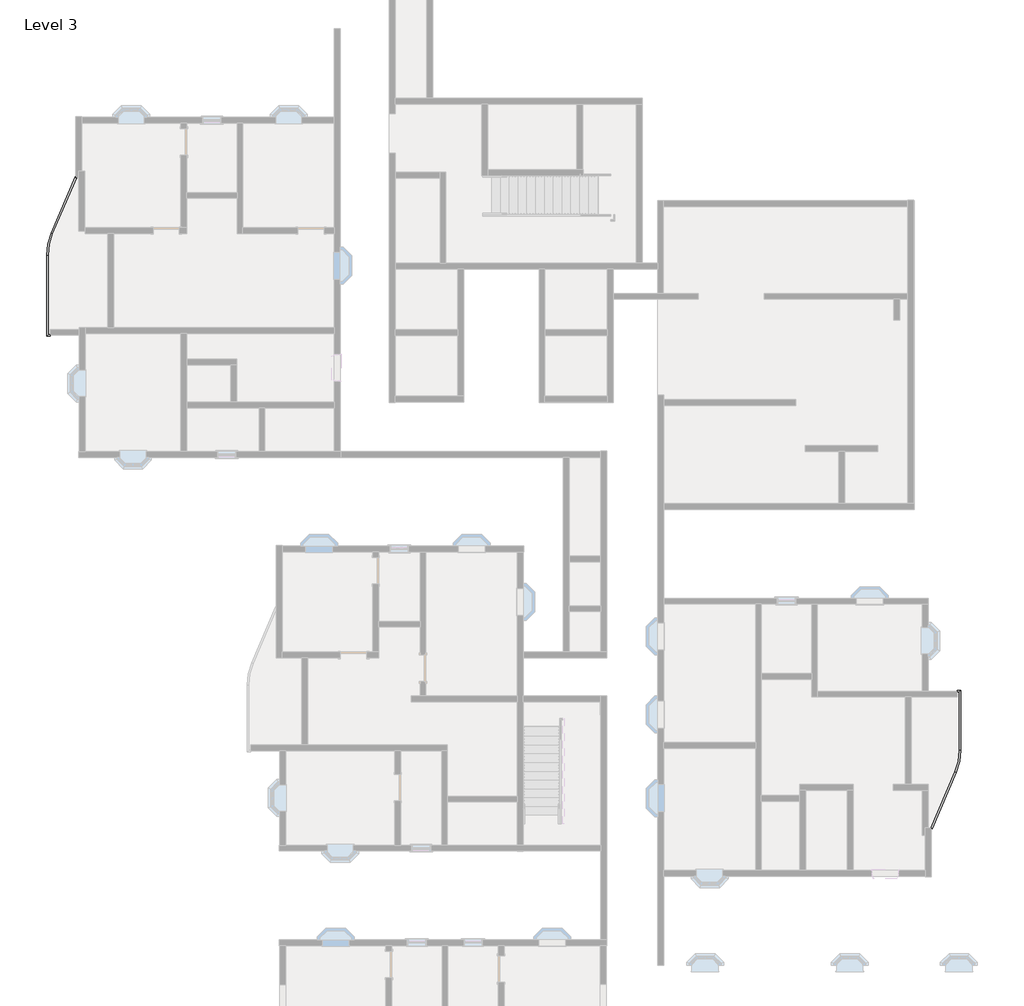
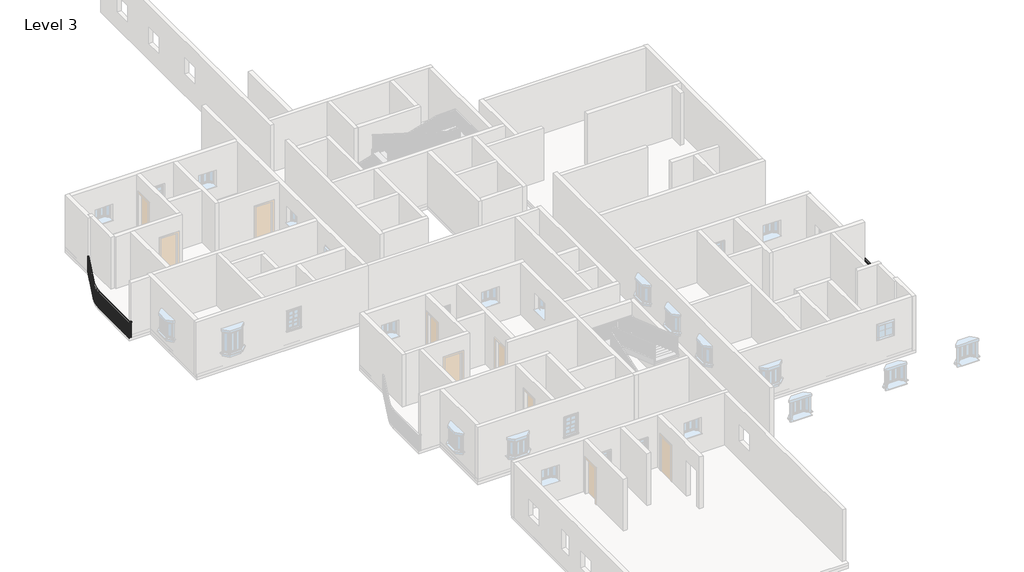
# One storey, part 9 of 14: 2 railings.
"""IFC4 building model written with IfcOpenShell, lengths in millimetres."""

from ifc_helpers import new_model, si_unit, frame, origin, place, context, project, spatial, polyline, circle_curve, outline, extrude, element, save
from ifc_brep_helpers import plane_surface, cylinder_surface, revolved_surface, advanced_brep

model = new_model("IFC4")

# Units and contexts
model_context = context("Model", 3, world=origin())
ifc_project = project(units=[si_unit("LENGTHUNIT", "METRE", prefix="MILLI")], contexts=[model_context])

# Site, building, storey
site = spatial("IfcSite", under=ifc_project)
building = spatial("IfcBuilding", under=site)
storey = spatial("IfcBuildingStorey", under=building, Name="Level 3", Elevation=6096.0)

# Railings
placement = place(None, origin())
element("IfcRailing", 1, ObjectType="Handrail - Rectangular", at=placement, inside=storey, context=model_context, shape_type="SolidModel", body=[
    advanced_brep(
    [(-19327.739878, 12446.0257339, 7010.4), (-19327.739878, 12446.0257339, 6959.6), (-19374.4383922, 12466.022953, 6959.6), (-19374.4383922, 12466.022953, 7010.4), (-20162.483418, 10496.6905323, 7010.4), (-20162.483418, 10496.6905323, 6959.6), (-20209.1819322, 10516.6877514, 6959.6), (-20209.1819322, 10516.6877514, 7010.4), (-20316.2891351, 9746.7948172, 6959.6), (-20316.2891351, 9746.7948172, 7010.4), (-20367.0891351, 9746.7948172, 6959.6), (-20367.0891351, 9746.7948172, 7010.4), (-20316.2891351, 7005.2583494, 7010.4), (-20316.2891351, 7005.2583494, 6959.6), (-20367.0891351, 6954.4583494, 6959.6), (-20367.0891351, 6954.4583494, 7010.4), (-20240.0891351, 7005.2583494, 7010.4), (-20240.0891351, 6954.4583494, 7010.4), (-20240.0891351, 6954.4583494, 6959.6), (-20240.0891351, 7005.2583494, 6959.6)],
    [
        (0, 1),
        (1, 2),
        (2, 3),
        (3, 0),
        (0, 4),
        (4, 5),
        (5, 1),
        (5, 6),
        (6, 2),
        (6, 7),
        (7, 3),
        (7, 4),
        (8, 5, circle_curve(frame((-18411.2891351, 9746.7948172, 6959.6), z_axis=(0.0, 0.0, -1.0), x_axis=(-0.919262090762392, 0.3936460446735823, 0.0)), 1905.0)),
        (4, 9, circle_curve(frame((-18411.2891351, 9746.7948172, 7010.4), z_axis=(0.0, 0.0, 1.0), x_axis=(-0.919262090762392, 0.3936460446735823, 0.0)), 1905.0)),
        (9, 8),
        (10, 6, circle_curve(frame((-18411.2891351, 9746.7948172, 6959.6), z_axis=(0.0, 0.0, -1.0), x_axis=(-0.919262090762392, 0.3936460446735823, 0.0)), 1955.8)),
        (8, 10),
        (11, 7, circle_curve(frame((-18411.2891351, 9746.7948172, 7010.4), z_axis=(0.0, 0.0, -1.0), x_axis=(-0.919262090762392, 0.3936460446735823, 0.0)), 1955.8)),
        (10, 11),
        (11, 9),
        (9, 12),
        (12, 13),
        (13, 8),
        (13, 14),
        (14, 10),
        (14, 15),
        (15, 11),
        (15, 12),
        (16, 17),
        (17, 18),
        (18, 19),
        (19, 16),
        (12, 16),
        (19, 13),
        (18, 14),
        (17, 15),
    ],
    [
        plane_surface(frame((-19351.0891351, 12456.0243434, 7010.4), z_axis=(0.3936460446735829, 0.9192620907623917, 0.0), x_axis=(0.9192620907623917, -0.3936460446735829, 0.0))),
        plane_surface(frame((-19327.739878, 12446.0257339, 7010.4), z_axis=(0.9192620907623915, -0.3936460446735834, 0.0), x_axis=(-0.3936460446735834, -0.9192620907623915, 0.0))),
        plane_surface(frame((-19327.739878, 12446.0257339, 6959.6), z_axis=(0.0, 0.0, -1.0000000000000002), x_axis=(-0.3936460446735834, -0.9192620907623915, 0.0))),
        plane_surface(frame((-19374.4383922, 12466.022953, 6959.6), z_axis=(-0.9192620907623916, 0.393646044673583, 0.0), x_axis=(-0.393646044673583, -0.9192620907623916, 0.0))),
        plane_surface(frame((-19374.4383922, 12466.022953, 7010.4), z_axis=(0.0, 0.0, 1.0), x_axis=(-0.393646044673583, -0.9192620907623916, 0.0))),
        revolved_surface(polyline([(-20162.483418002357, 10496.690532303173, 7010.4), (-20162.483418002357, 10496.690532303173, 6959.6)]), (-18411.2891351, 9746.7948172, 7010.4), (0.0, 0.0, 1.0)),
        plane_surface(frame((-18411.2891351, 9746.7948172, 6959.6), z_axis=(0.0, 0.0, -1.0), x_axis=(-0.919262090762392, 0.3936460446735823, 0.0))),
        cylinder_surface(frame((-18411.2891351, 9746.7948172, 7010.4), z_axis=(0.0, 0.0, 1.0), x_axis=(-0.919262090762392, 0.3936460446735823, 0.0)), 1955.8),
        plane_surface(frame((-18411.2891351, 9746.7948172, 7010.4), z_axis=(0.0, 0.0, 1.0), x_axis=(-0.919262090762392, 0.3936460446735823, 0.0))),
        plane_surface(frame((-20316.2891351, 9746.7948172, 7010.4), z_axis=(1.0, 0.0, 0.0), x_axis=(0.0, -1.0, 0.0))),
        plane_surface(frame((-20316.2891351, 9746.7948172, 6959.6), z_axis=(0.0, 0.0, -1.0), x_axis=(0.0, -1.0, 0.0))),
        plane_surface(frame((-20367.0891351, 9746.7948172, 6959.6), z_axis=(-1.0, 0.0, 0.0), x_axis=(0.0, -1.0, 0.0))),
        plane_surface(frame((-20367.0891351, 9746.7948172, 7010.4), z_axis=(0.0, 0.0, 1.0), x_axis=(0.0, -1.0, 0.0))),
        plane_surface(frame((-20240.0891351, 6979.8583494, 7010.4), z_axis=(1.0, 0.0, 0.0), x_axis=(0.0, 1.0, 0.0))),
        plane_surface(frame((-20316.2891351, 7005.2583494, 7010.4), z_axis=(0.0, 1.0, 0.0), x_axis=(1.0, 0.0, 0.0))),
        plane_surface(frame((-20316.2891351, 7005.2583494, 6959.6), z_axis=(0.0, 0.0, -1.0), x_axis=(1.0, 0.0, 0.0))),
        plane_surface(frame((-20367.0891351, 6954.4583494, 6959.6), z_axis=(0.0, -1.0, 0.0), x_axis=(1.0, 0.0, 0.0))),
        plane_surface(frame((-20367.0891351, 6954.4583494, 7010.4), z_axis=(0.0, 0.0, 1.0), x_axis=(1.0, 0.0, 0.0))),
    ],
    [
        (0, [[1, 2, 3, 4]]),
        (1, [[-1, 5, 6, 7]]),
        (2, [[-2, -7, 8, 9]]),
        (3, [[-3, -9, 10, 11]]),
        (4, [[-4, -11, 12, -5]]),
        (5, [[13, -6, 14, 15]]),
        (6, [[16, -8, -13, 17]]),
        (7, [[18, -10, -16, 19]]),
        (8, [[-14, -12, -18, 20]]),
        (9, [[-15, 21, 22, 23]]),
        (10, [[-17, -23, 24, 25]]),
        (11, [[-19, -25, 26, 27]]),
        (12, [[-20, -27, 28, -21]]),
        (13, [[29, 30, 31, 32]]),
        (14, [[-22, 33, -32, 34]]),
        (15, [[-24, -34, -31, 35]]),
        (16, [[-26, -35, -30, 36]]),
        (17, [[-28, -36, -29, -33]]),
    ],
),
    extrude(outline(polyline([(-20351.2141351, 7013.1198172), (-20332.1641351, 7013.1198172), (-20332.1641351, 6994.0698172), (-20351.2141351, 6994.0698172), (-20351.2141351, 7013.1198172)])), frame((0.0, 0.0, 6096.0), z_axis=(0.0, 0.0, 1.0), x_axis=(1.0, 0.0, 0.0)), (0.0, 0.0, 1.0), 863.6),
    extrude(outline(polyline([(-20351.2141351, 7114.7198172), (-20332.1641351, 7114.7198172), (-20332.1641351, 7095.6698172), (-20351.2141351, 7095.6698172), (-20351.2141351, 7114.7198172)])), frame((0.0, 0.0, 6096.0), z_axis=(0.0, 0.0, 1.0), x_axis=(1.0, 0.0, 0.0)), (0.0, 0.0, 1.0), 863.6),
    extrude(outline(polyline([(-20351.2141351, 7216.3198172), (-20332.1641351, 7216.3198172), (-20332.1641351, 7197.2698172), (-20351.2141351, 7197.2698172), (-20351.2141351, 7216.3198172)])), frame((0.0, 0.0, 6096.0), z_axis=(0.0, 0.0, 1.0), x_axis=(1.0, 0.0, 0.0)), (0.0, 0.0, 1.0), 863.6),
    extrude(outline(polyline([(-20351.2141351, 7317.9198172), (-20332.1641351, 7317.9198172), (-20332.1641351, 7298.8698172), (-20351.2141351, 7298.8698172), (-20351.2141351, 7317.9198172)])), frame((0.0, 0.0, 6096.0), z_axis=(0.0, 0.0, 1.0), x_axis=(1.0, 0.0, 0.0)), (0.0, 0.0, 1.0), 863.6),
    extrude(outline(polyline([(-20351.2141351, 7419.5198172), (-20332.1641351, 7419.5198172), (-20332.1641351, 7400.4698172), (-20351.2141351, 7400.4698172), (-20351.2141351, 7419.5198172)])), frame((0.0, 0.0, 6096.0), z_axis=(0.0, 0.0, 1.0), x_axis=(1.0, 0.0, 0.0)), (0.0, 0.0, 1.0), 863.6),
    extrude(outline(polyline([(-20351.2141351, 7521.1198172), (-20332.1641351, 7521.1198172), (-20332.1641351, 7502.0698172), (-20351.2141351, 7502.0698172), (-20351.2141351, 7521.1198172)])), frame((0.0, 0.0, 6096.0), z_axis=(0.0, 0.0, 1.0), x_axis=(1.0, 0.0, 0.0)), (0.0, 0.0, 1.0), 863.6),
    extrude(outline(polyline([(-20351.2141351, 7622.7198172), (-20332.1641351, 7622.7198172), (-20332.1641351, 7603.6698172), (-20351.2141351, 7603.6698172), (-20351.2141351, 7622.7198172)])), frame((0.0, 0.0, 6096.0), z_axis=(0.0, 0.0, 1.0), x_axis=(1.0, 0.0, 0.0)), (0.0, 0.0, 1.0), 863.6),
    extrude(outline(polyline([(-20351.2141351, 7724.3198172), (-20332.1641351, 7724.3198172), (-20332.1641351, 7705.2698172), (-20351.2141351, 7705.2698172), (-20351.2141351, 7724.3198172)])), frame((0.0, 0.0, 6096.0), z_axis=(0.0, 0.0, 1.0), x_axis=(1.0, 0.0, 0.0)), (0.0, 0.0, 1.0), 863.6),
    extrude(outline(polyline([(-20351.2141351, 7825.9198172), (-20332.1641351, 7825.9198172), (-20332.1641351, 7806.8698172), (-20351.2141351, 7806.8698172), (-20351.2141351, 7825.9198172)])), frame((0.0, 0.0, 6096.0), z_axis=(0.0, 0.0, 1.0), x_axis=(1.0, 0.0, 0.0)), (0.0, 0.0, 1.0), 863.6),
    extrude(outline(polyline([(-20351.2141351, 7927.5198172), (-20332.1641351, 7927.5198172), (-20332.1641351, 7908.4698172), (-20351.2141351, 7908.4698172), (-20351.2141351, 7927.5198172)])), frame((0.0, 0.0, 6096.0), z_axis=(0.0, 0.0, 1.0), x_axis=(1.0, 0.0, 0.0)), (0.0, 0.0, 1.0), 863.6),
    extrude(outline(polyline([(-20351.2141351, 8029.1198172), (-20332.1641351, 8029.1198172), (-20332.1641351, 8010.0698172), (-20351.2141351, 8010.0698172), (-20351.2141351, 8029.1198172)])), frame((0.0, 0.0, 6096.0), z_axis=(0.0, 0.0, 1.0), x_axis=(1.0, 0.0, 0.0)), (0.0, 0.0, 1.0), 863.6),
    extrude(outline(polyline([(-20351.2141351, 8130.7198172), (-20332.1641351, 8130.7198172), (-20332.1641351, 8111.6698172), (-20351.2141351, 8111.6698172), (-20351.2141351, 8130.7198172)])), frame((0.0, 0.0, 6096.0), z_axis=(0.0, 0.0, 1.0), x_axis=(1.0, 0.0, 0.0)), (0.0, 0.0, 1.0), 863.6),
    extrude(outline(polyline([(-20351.2141351, 8232.3198172), (-20332.1641351, 8232.3198172), (-20332.1641351, 8213.2698172), (-20351.2141351, 8213.2698172), (-20351.2141351, 8232.3198172)])), frame((0.0, 0.0, 6096.0), z_axis=(0.0, 0.0, 1.0), x_axis=(1.0, 0.0, 0.0)), (0.0, 0.0, 1.0), 863.6),
    extrude(outline(polyline([(-20351.2141351, 8333.9198172), (-20332.1641351, 8333.9198172), (-20332.1641351, 8314.8698172), (-20351.2141351, 8314.8698172), (-20351.2141351, 8333.9198172)])), frame((0.0, 0.0, 6096.0), z_axis=(0.0, 0.0, 1.0), x_axis=(1.0, 0.0, 0.0)), (0.0, 0.0, 1.0), 863.6),
    extrude(outline(polyline([(-20351.2141351, 8435.5198172), (-20332.1641351, 8435.5198172), (-20332.1641351, 8416.4698172), (-20351.2141351, 8416.4698172), (-20351.2141351, 8435.5198172)])), frame((0.0, 0.0, 6096.0), z_axis=(0.0, 0.0, 1.0), x_axis=(1.0, 0.0, 0.0)), (0.0, 0.0, 1.0), 863.6),
    extrude(outline(polyline([(-20351.2141351, 8537.1198172), (-20332.1641351, 8537.1198172), (-20332.1641351, 8518.0698172), (-20351.2141351, 8518.0698172), (-20351.2141351, 8537.1198172)])), frame((0.0, 0.0, 6096.0), z_axis=(0.0, 0.0, 1.0), x_axis=(1.0, 0.0, 0.0)), (0.0, 0.0, 1.0), 863.6),
    extrude(outline(polyline([(-20351.2141351, 8638.7198172), (-20332.1641351, 8638.7198172), (-20332.1641351, 8619.6698172), (-20351.2141351, 8619.6698172), (-20351.2141351, 8638.7198172)])), frame((0.0, 0.0, 6096.0), z_axis=(0.0, 0.0, 1.0), x_axis=(1.0, 0.0, 0.0)), (0.0, 0.0, 1.0), 863.6),
    extrude(outline(polyline([(-20351.2141351, 8740.3198172), (-20332.1641351, 8740.3198172), (-20332.1641351, 8721.2698172), (-20351.2141351, 8721.2698172), (-20351.2141351, 8740.3198172)])), frame((0.0, 0.0, 6096.0), z_axis=(0.0, 0.0, 1.0), x_axis=(1.0, 0.0, 0.0)), (0.0, 0.0, 1.0), 863.6),
    extrude(outline(polyline([(-20351.2141351, 8841.9198172), (-20332.1641351, 8841.9198172), (-20332.1641351, 8822.8698172), (-20351.2141351, 8822.8698172), (-20351.2141351, 8841.9198172)])), frame((0.0, 0.0, 6096.0), z_axis=(0.0, 0.0, 1.0), x_axis=(1.0, 0.0, 0.0)), (0.0, 0.0, 1.0), 863.6),
    extrude(outline(polyline([(-20351.2141351, 8943.5198172), (-20332.1641351, 8943.5198172), (-20332.1641351, 8924.4698172), (-20351.2141351, 8924.4698172), (-20351.2141351, 8943.5198172)])), frame((0.0, 0.0, 6096.0), z_axis=(0.0, 0.0, 1.0), x_axis=(1.0, 0.0, 0.0)), (0.0, 0.0, 1.0), 863.6),
    extrude(outline(polyline([(-20351.2141351, 9045.1198172), (-20332.1641351, 9045.1198172), (-20332.1641351, 9026.0698172), (-20351.2141351, 9026.0698172), (-20351.2141351, 9045.1198172)])), frame((0.0, 0.0, 6096.0), z_axis=(0.0, 0.0, 1.0), x_axis=(1.0, 0.0, 0.0)), (0.0, 0.0, 1.0), 863.6),
    extrude(outline(polyline([(-20351.2141351, 9146.7198172), (-20332.1641351, 9146.7198172), (-20332.1641351, 9127.6698172), (-20351.2141351, 9127.6698172), (-20351.2141351, 9146.7198172)])), frame((0.0, 0.0, 6096.0), z_axis=(0.0, 0.0, 1.0), x_axis=(1.0, 0.0, 0.0)), (0.0, 0.0, 1.0), 863.6),
    extrude(outline(polyline([(-20351.2141351, 9248.3198172), (-20332.1641351, 9248.3198172), (-20332.1641351, 9229.2698172), (-20351.2141351, 9229.2698172), (-20351.2141351, 9248.3198172)])), frame((0.0, 0.0, 6096.0), z_axis=(0.0, 0.0, 1.0), x_axis=(1.0, 0.0, 0.0)), (0.0, 0.0, 1.0), 863.6),
    extrude(outline(polyline([(-20351.2141351, 9349.9198172), (-20332.1641351, 9349.9198172), (-20332.1641351, 9330.8698172), (-20351.2141351, 9330.8698172), (-20351.2141351, 9349.9198172)])), frame((0.0, 0.0, 6096.0), z_axis=(0.0, 0.0, 1.0), x_axis=(1.0, 0.0, 0.0)), (0.0, 0.0, 1.0), 863.6),
    extrude(outline(polyline([(-20351.2141351, 9451.5198172), (-20332.1641351, 9451.5198172), (-20332.1641351, 9432.4698172), (-20351.2141351, 9432.4698172), (-20351.2141351, 9451.5198172)])), frame((0.0, 0.0, 6096.0), z_axis=(0.0, 0.0, 1.0), x_axis=(1.0, 0.0, 0.0)), (0.0, 0.0, 1.0), 863.6),
    extrude(outline(polyline([(-20351.2141351, 9553.1198172), (-20332.1641351, 9553.1198172), (-20332.1641351, 9534.0698172), (-20351.2141351, 9534.0698172), (-20351.2141351, 9553.1198172)])), frame((0.0, 0.0, 6096.0), z_axis=(0.0, 0.0, 1.0), x_axis=(1.0, 0.0, 0.0)), (0.0, 0.0, 1.0), 863.6),
    extrude(outline(polyline([(-20351.2141351, 9654.7198172), (-20332.1641351, 9654.7198172), (-20332.1641351, 9635.6698172), (-20351.2141351, 9635.6698172), (-20351.2141351, 9654.7198172)])), frame((0.0, 0.0, 6096.0), z_axis=(0.0, 0.0, 1.0), x_axis=(1.0, 0.0, 0.0)), (0.0, 0.0, 1.0), 863.6),
    extrude(outline(polyline([(-20349.6005818, 9826.4720848), (-20330.5630441, 9825.7831307), (-20331.2519982, 9806.745593), (-20350.289536, 9807.4345471), (-20349.6005818, 9826.4720848)])), frame((0.0, 0.0, 6096.0), z_axis=(0.0, 0.0, 1.0), x_axis=(1.0, 0.0, 0.0)), (0.0, 0.0, 1.0), 863.6),
    extrude(outline(polyline([(-20342.724955, 9928.3310534), (-20323.750023, 9926.6415402), (-20325.4395363, 9907.6666081), (-20344.4144683, 9909.3561214), (-20342.724955, 9928.3310534)])), frame((0.0, 0.0, 6096.0), z_axis=(0.0, 0.0, 1.0), x_axis=(1.0, 0.0, 0.0)), (0.0, 0.0, 1.0), 863.6),
    extrude(outline(polyline([(-20330.5003254, 10029.6872677), (-20311.6405491, 10027.0018743), (-20314.3259425, 10008.142098), (-20333.1857188, 10010.8274914), (-20330.5003254, 10029.6872677)])), frame((0.0, 0.0, 6096.0), z_axis=(0.0, 0.0, 1.0), x_axis=(1.0, 0.0, 0.0)), (0.0, 0.0, 1.0), 863.6),
    extrude(outline(polyline([(-20312.9605484, 10130.2600272), (-20294.2681589, 10126.5861907), (-20297.9419954, 10107.8938012), (-20316.6343849, 10111.5676377), (-20312.9605484, 10130.2600272)])), frame((0.0, 0.0, 6096.0), z_axis=(0.0, 0.0, 1.0), x_axis=(1.0, 0.0, 0.0)), (0.0, 0.0, 1.0), 863.6),
    extrude(outline(polyline([(-20290.1541995, 10229.7708014), (-20271.6809643, 10225.1186963), (-20276.3330693, 10206.6454611), (-20294.8063045, 10211.2975662), (-20290.1541995, 10229.7708014)])), frame((0.0, 0.0, 6096.0), z_axis=(0.0, 0.0, 1.0), x_axis=(1.0, 0.0, 0.0)), (0.0, 0.0, 1.0), 863.6),
    extrude(outline(polyline([(-20262.1444395, 10327.9440008), (-20243.9415192, 10322.3265109), (-20249.5590091, 10304.1235906), (-20267.7619294, 10309.7410805), (-20262.1444395, 10327.9440008)])), frame((0.0, 0.0, 6096.0), z_axis=(0.0, 0.0, 1.0), x_axis=(1.0, 0.0, 0.0)), (0.0, 0.0, 1.0), 863.6),
    extrude(outline(polyline([(-20229.0088399, 10424.5077402), (-20211.1266465, 10417.9404228), (-20217.693964, 10400.0582293), (-20235.5761574, 10406.6255468), (-20229.0088399, 10424.5077402)])), frame((0.0, 0.0, 6096.0), z_axis=(0.0, 0.0, 1.0), x_axis=(1.0, 0.0, 0.0)), (0.0, 0.0, 1.0), 863.6),
    extrude(outline(polyline([(-20155.9843907, 10600.589225), (-20138.4724479, 10593.0902678), (-20145.9714051, 10575.578325), (-20163.4833479, 10583.0772822), (-20155.9843907, 10600.589225)])), frame((0.0, 0.0, 6096.0), z_axis=(0.0, 0.0, 1.0), x_axis=(1.0, 0.0, 0.0)), (0.0, 0.0, 1.0), 863.6),
    extrude(outline(polyline([(-20115.9899526, 10693.9862534), (-20098.4780098, 10686.4872963), (-20105.9769669, 10668.9753534), (-20123.4889098, 10676.4743106), (-20115.9899526, 10693.9862534)])), frame((0.0, 0.0, 6096.0), z_axis=(0.0, 0.0, 1.0), x_axis=(1.0, 0.0, 0.0)), (0.0, 0.0, 1.0), 863.6),
    extrude(outline(polyline([(-20075.9955145, 10787.3832818), (-20058.4835716, 10779.8843247), (-20065.9825288, 10762.3723818), (-20083.4944716, 10769.871339), (-20075.9955145, 10787.3832818)])), frame((0.0, 0.0, 6096.0), z_axis=(0.0, 0.0, 1.0), x_axis=(1.0, 0.0, 0.0)), (0.0, 0.0, 1.0), 863.6),
    extrude(outline(polyline([(-20036.0010763, 10880.7803103), (-20018.4891335, 10873.2813531), (-20025.9880906, 10855.7694103), (-20043.5000335, 10863.2683674), (-20036.0010763, 10880.7803103)])), frame((0.0, 0.0, 6096.0), z_axis=(0.0, 0.0, 1.0), x_axis=(1.0, 0.0, 0.0)), (0.0, 0.0, 1.0), 863.6),
    extrude(outline(polyline([(-19996.0066382, 10974.1773387), (-19978.4946954, 10966.6783815), (-19985.9936525, 10949.1664387), (-20003.5055953, 10956.6653958), (-19996.0066382, 10974.1773387)])), frame((0.0, 0.0, 6096.0), z_axis=(0.0, 0.0, 1.0), x_axis=(1.0, 0.0, 0.0)), (0.0, 0.0, 1.0), 863.6),
    extrude(outline(polyline([(-19956.0122, 11067.5743671), (-19938.5002572, 11060.0754099), (-19945.9992144, 11042.5634671), (-19963.5111572, 11050.0624243), (-19956.0122, 11067.5743671)])), frame((0.0, 0.0, 6096.0), z_axis=(0.0, 0.0, 1.0), x_axis=(1.0, 0.0, 0.0)), (0.0, 0.0, 1.0), 863.6),
    extrude(outline(polyline([(-19916.0177619, 11160.9713955), (-19898.5058191, 11153.4724384), (-19906.0047762, 11135.9604955), (-19923.5167191, 11143.4594527), (-19916.0177619, 11160.9713955)])), frame((0.0, 0.0, 6096.0), z_axis=(0.0, 0.0, 1.0), x_axis=(1.0, 0.0, 0.0)), (0.0, 0.0, 1.0), 863.6),
    extrude(outline(polyline([(-19876.0233238, 11254.3684239), (-19858.5113809, 11246.8694668), (-19866.0103381, 11229.357524), (-19883.5222809, 11236.8564811), (-19876.0233238, 11254.3684239)])), frame((0.0, 0.0, 6096.0), z_axis=(0.0, 0.0, 1.0), x_axis=(1.0, 0.0, 0.0)), (0.0, 0.0, 1.0), 863.6),
    extrude(outline(polyline([(-19836.0288856, 11347.7654524), (-19818.5169428, 11340.2664952), (-19826.0159, 11322.7545524), (-19843.5278428, 11330.2535095), (-19836.0288856, 11347.7654524)])), frame((0.0, 0.0, 6096.0), z_axis=(0.0, 0.0, 1.0), x_axis=(1.0, 0.0, 0.0)), (0.0, 0.0, 1.0), 863.6),
    extrude(outline(polyline([(-19796.0344475, 11441.1624808), (-19778.5225047, 11433.6635236), (-19786.0214618, 11416.1515808), (-19803.5334046, 11423.650538), (-19796.0344475, 11441.1624808)])), frame((0.0, 0.0, 6096.0), z_axis=(0.0, 0.0, 1.0), x_axis=(1.0, 0.0, 0.0)), (0.0, 0.0, 1.0), 863.6),
    extrude(outline(polyline([(-19756.0400094, 11534.5595092), (-19738.5280665, 11527.060552), (-19746.0270237, 11509.5486092), (-19763.5389665, 11517.0475664), (-19756.0400094, 11534.5595092)])), frame((0.0, 0.0, 6096.0), z_axis=(0.0, 0.0, 1.0), x_axis=(1.0, 0.0, 0.0)), (0.0, 0.0, 1.0), 863.6),
    extrude(outline(polyline([(-19716.0455712, 11627.9565376), (-19698.5336284, 11620.4575805), (-19706.0325855, 11602.9456376), (-19723.5445284, 11610.4445948), (-19716.0455712, 11627.9565376)])), frame((0.0, 0.0, 6096.0), z_axis=(0.0, 0.0, 1.0), x_axis=(1.0, 0.0, 0.0)), (0.0, 0.0, 1.0), 863.6),
    extrude(outline(polyline([(-19676.0511331, 11721.353566), (-19658.5391902, 11713.8546089), (-19666.0381474, 11696.3426661), (-19683.5500902, 11703.8416232), (-19676.0511331, 11721.353566)])), frame((0.0, 0.0, 6096.0), z_axis=(0.0, 0.0, 1.0), x_axis=(1.0, 0.0, 0.0)), (0.0, 0.0, 1.0), 863.6),
    extrude(outline(polyline([(-19636.0566949, 11814.7505945), (-19618.5447521, 11807.2516373), (-19626.0437093, 11789.7396945), (-19643.5556521, 11797.2386516), (-19636.0566949, 11814.7505945)])), frame((0.0, 0.0, 6096.0), z_axis=(0.0, 0.0, 1.0), x_axis=(1.0, 0.0, 0.0)), (0.0, 0.0, 1.0), 863.6),
    extrude(outline(polyline([(-19596.0622568, 11908.1476229), (-19578.550314, 11900.6486657), (-19586.0492711, 11883.1367229), (-19603.561214, 11890.6356801), (-19596.0622568, 11908.1476229)])), frame((0.0, 0.0, 6096.0), z_axis=(0.0, 0.0, 1.0), x_axis=(1.0, 0.0, 0.0)), (0.0, 0.0, 1.0), 863.6),
    extrude(outline(polyline([(-19556.0678187, 12001.5446513), (-19538.5558758, 11994.0456942), (-19546.054833, 11976.5337513), (-19563.5667758, 11984.0327085), (-19556.0678187, 12001.5446513)])), frame((0.0, 0.0, 6096.0), z_axis=(0.0, 0.0, 1.0), x_axis=(1.0, 0.0, 0.0)), (0.0, 0.0, 1.0), 863.6),
    extrude(outline(polyline([(-19516.0733805, 12094.9416797), (-19498.5614377, 12087.4427226), (-19506.0603948, 12069.9307797), (-19523.5723377, 12077.4297369), (-19516.0733805, 12094.9416797)])), frame((0.0, 0.0, 6096.0), z_axis=(0.0, 0.0, 1.0), x_axis=(1.0, 0.0, 0.0)), (0.0, 0.0, 1.0), 863.6),
    extrude(outline(polyline([(-19476.0789424, 12188.3387082), (-19458.5669996, 12180.839751), (-19466.0659567, 12163.3278082), (-19483.5778995, 12170.8267653), (-19476.0789424, 12188.3387082)])), frame((0.0, 0.0, 6096.0), z_axis=(0.0, 0.0, 1.0), x_axis=(1.0, 0.0, 0.0)), (0.0, 0.0, 1.0), 863.6),
    extrude(outline(polyline([(-19436.0845042, 12281.7357366), (-19418.5725614, 12274.2367794), (-19426.0715186, 12256.7248366), (-19443.5834614, 12264.2237937), (-19436.0845042, 12281.7357366)])), frame((0.0, 0.0, 6096.0), z_axis=(0.0, 0.0, 1.0), x_axis=(1.0, 0.0, 0.0)), (0.0, 0.0, 1.0), 863.6),
    extrude(outline(polyline([(-19396.0900661, 12375.132765), (-19378.5781233, 12367.6338078), (-19386.0770804, 12350.121865), (-19403.5890233, 12357.6208222), (-19396.0900661, 12375.132765)])), frame((0.0, 0.0, 6096.0), z_axis=(0.0, 0.0, 1.0), x_axis=(1.0, 0.0, 0.0)), (0.0, 0.0, 1.0), 863.6),
    extrude(outline(polyline([(-20351.2141351, 6989.3833494), (-20332.1641351, 6989.3833494), (-20332.1641351, 6970.3333494), (-20351.2141351, 6970.3333494), (-20351.2141351, 6989.3833494)])), frame((0.0, 0.0, 6096.0), z_axis=(0.0, 0.0, 1.0), x_axis=(1.0, 0.0, 0.0)), (0.0, 0.0, 1.0), 863.6),
    extrude(outline(polyline([(-20351.2141351, 9756.3198172), (-20332.1641351, 9756.3198172), (-20332.1641351, 9737.2698172), (-20351.2141351, 9737.2698172), (-20351.2141351, 9756.3198172)])), frame((0.0, 0.0, 6096.0), z_axis=(0.0, 0.0, 1.0), x_axis=(1.0, 0.0, 0.0)), (0.0, 0.0, 1.0), 863.6),
    extrude(outline(polyline([(-20190.839168, 10519.1945919), (-20173.3272251, 10511.6956347), (-20180.8261823, 10494.1836919), (-20198.3381251, 10501.682649), (-20190.839168, 10519.1945919)])), frame((0.0, 0.0, 6096.0), z_axis=(0.0, 0.0, 1.0), x_axis=(1.0, 0.0, 0.0)), (0.0, 0.0, 1.0), 863.6),
    extrude(outline(polyline([(-20259.1391351, 6970.3333494), (-20259.1391351, 6989.3833494), (-20240.0891351, 6989.3833494), (-20240.0891351, 6970.3333494), (-20259.1391351, 6970.3333494)])), frame((0.0, 0.0, 6096.0), z_axis=(0.0, 0.0, 1.0), x_axis=(1.0, 0.0, 0.0)), (0.0, 0.0, 1.0), 863.6),
    extrude(outline(polyline([(-19359.8451065, 12459.773822), (-19342.3331637, 12452.2748648), (-19349.8321209, 12434.762922), (-19367.3440637, 12442.2618792), (-19359.8451065, 12459.773822)])), frame((0.0, 0.0, 6096.0), z_axis=(0.0, 0.0, 1.0), x_axis=(1.0, 0.0, 0.0)), (0.0, 0.0, 1.0), 863.6),
])
element("IfcRailing", 2, ObjectType="Handrail - Rectangular", at=placement, inside=storey, context=model_context, shape_type="SolidModel", body=[
    advanced_brep(
    [(10250.7887952, -10096.81198, 7010.4), (10250.7887952, -10096.81198, 6959.6), (10297.4873094, -10116.8091991, 6959.6), (10297.4873094, -10116.8091991, 7010.4), (11085.5323352, -8147.4767784, 7010.4), (11085.5323352, -8147.4767784, 6959.6), (11132.2308494, -8167.4739975, 6959.6), (11132.2308494, -8167.4739975, 7010.4), (11239.3380523, -7397.5810633, 6959.6), (11239.3380523, -7397.5810633, 7010.4), (11290.1380523, -7397.5810633, 6959.6), (11290.1380523, -7397.5810633, 7010.4), (11239.3380523, -5378.0542694, 7010.4), (11239.3380523, -5378.0542694, 6959.6), (11290.1380523, -5327.2542694, 6959.6), (11290.1380523, -5327.2542694, 7010.4), (11163.1380523, -5378.0542694, 7010.4), (11163.1380523, -5327.2542694, 7010.4), (11163.1380523, -5327.2542694, 6959.6), (11163.1380523, -5378.0542694, 6959.6)],
    [
        (0, 1),
        (1, 2),
        (2, 3),
        (3, 0),
        (0, 4),
        (4, 5),
        (5, 1),
        (5, 6),
        (6, 2),
        (6, 7),
        (7, 3),
        (7, 4),
        (8, 5, circle_curve(frame((9334.3380523, -7397.5810633, 6959.6), z_axis=(0.0, 0.0, -1.0), x_axis=(0.9192620907624003, -0.3936460446735628, 0.0)), 1905.0)),
        (4, 9, circle_curve(frame((9334.3380523, -7397.5810633, 7010.4), z_axis=(0.0, 0.0, 1.0), x_axis=(0.9192620907624003, -0.3936460446735628, 0.0)), 1905.0)),
        (9, 8),
        (10, 6, circle_curve(frame((9334.3380523, -7397.5810633, 6959.6), z_axis=(0.0, 0.0, -1.0), x_axis=(0.9192620907624003, -0.3936460446735628, 0.0)), 1955.8)),
        (8, 10),
        (11, 7, circle_curve(frame((9334.3380523, -7397.5810633, 7010.4), z_axis=(0.0, 0.0, -1.0), x_axis=(0.9192620907624003, -0.3936460446735628, 0.0)), 1955.8)),
        (10, 11),
        (11, 9),
        (9, 12),
        (12, 13),
        (13, 8),
        (13, 14),
        (14, 10),
        (14, 15),
        (15, 11),
        (15, 12),
        (16, 17),
        (17, 18),
        (18, 19),
        (19, 16),
        (12, 16),
        (19, 13),
        (18, 14),
        (17, 15),
    ],
    [
        plane_surface(frame((10274.1380523, -10106.8105895, 7010.4), z_axis=(-0.3936460446735629, -0.9192620907624003, 0.0), x_axis=(0.9192620907624003, -0.3936460446735629, 0.0))),
        plane_surface(frame((10250.7887952, -10096.81198, 7010.4), z_axis=(-0.9192620907624004, 0.3936460446735625, 0.0), x_axis=(0.3936460446735625, 0.9192620907624004, 0.0))),
        plane_surface(frame((10250.7887952, -10096.81198, 6959.6), z_axis=(0.0, 0.0, -1.0), x_axis=(0.3936460446735625, 0.9192620907624004, 0.0))),
        plane_surface(frame((10297.4873094, -10116.8091991, 6959.6), z_axis=(0.9192620907624003, -0.3936460446735629, 0.0), x_axis=(0.3936460446735629, 0.9192620907624003, 0.0))),
        plane_surface(frame((10297.4873094, -10116.8091991, 7010.4), z_axis=(0.0, 0.0, 1.0), x_axis=(0.3936460446735629, 0.9192620907624003, 0.0))),
        revolved_surface(polyline([(11085.532335202372, -8147.476778403137, 7010.4), (11085.532335202372, -8147.476778403137, 6959.6)]), (9334.3380523, -7397.5810633, 7010.4), (0.0, 0.0, 1.0)),
        plane_surface(frame((9334.3380523, -7397.5810633, 6959.6), z_axis=(0.0, 0.0, -1.0), x_axis=(0.9192620907624003, -0.3936460446735628, 0.0))),
        cylinder_surface(frame((9334.3380523, -7397.5810633, 7010.4), z_axis=(0.0, 0.0, 1.0), x_axis=(0.9192620907624003, -0.3936460446735628, 0.0)), 1955.8),
        plane_surface(frame((9334.3380523, -7397.5810633, 7010.4), z_axis=(0.0, 0.0, 1.0), x_axis=(0.9192620907624003, -0.3936460446735628, 0.0))),
        plane_surface(frame((11239.3380523, -7397.5810633, 7010.4), z_axis=(-1.0, 0.0, 0.0), x_axis=(0.0, 1.0, 0.0))),
        plane_surface(frame((11239.3380523, -7397.5810633, 6959.6), z_axis=(0.0, 0.0, -1.0), x_axis=(0.0, 1.0, 0.0))),
        plane_surface(frame((11290.1380523, -7397.5810633, 6959.6), z_axis=(1.0, 0.0, 0.0), x_axis=(0.0, 1.0, 0.0))),
        plane_surface(frame((11290.1380523, -7397.5810633, 7010.4), z_axis=(0.0, 0.0, 1.0), x_axis=(0.0, 1.0, 0.0))),
        plane_surface(frame((11163.1380523, -5352.6542694, 7010.4), z_axis=(-1.0, 0.0, 0.0), x_axis=(0.0, -1.0, 0.0))),
        plane_surface(frame((11239.3380523, -5378.0542694, 7010.4), z_axis=(0.0, -1.0, 0.0), x_axis=(-1.0, 0.0, 0.0))),
        plane_surface(frame((11239.3380523, -5378.0542694, 6959.6), z_axis=(0.0, 0.0, -1.0), x_axis=(-1.0, 0.0, 0.0))),
        plane_surface(frame((11290.1380523, -5327.2542694, 6959.6), z_axis=(0.0, 1.0, 0.0), x_axis=(-1.0, 0.0, 0.0))),
        plane_surface(frame((11290.1380523, -5327.2542694, 7010.4), z_axis=(0.0, 0.0, 1.0), x_axis=(-1.0, 0.0, 0.0))),
    ],
    [
        (0, [[1, 2, 3, 4]]),
        (1, [[-1, 5, 6, 7]]),
        (2, [[-2, -7, 8, 9]]),
        (3, [[-3, -9, 10, 11]]),
        (4, [[-4, -11, 12, -5]]),
        (5, [[13, -6, 14, 15]]),
        (6, [[16, -8, -13, 17]]),
        (7, [[18, -10, -16, 19]]),
        (8, [[-14, -12, -18, 20]]),
        (9, [[-15, 21, 22, 23]]),
        (10, [[-17, -23, 24, 25]]),
        (11, [[-19, -25, 26, 27]]),
        (12, [[-20, -27, 28, -21]]),
        (13, [[29, 30, 31, 32]]),
        (14, [[-22, 33, -32, 34]]),
        (15, [[-24, -34, -31, 35]]),
        (16, [[-26, -35, -30, 36]]),
        (17, [[-28, -36, -29, -33]]),
    ],
),
    extrude(outline(polyline([(11274.2630523, -5375.1060633), (11255.2130523, -5375.1060633), (11255.2130523, -5356.0560633), (11274.2630523, -5356.0560633), (11274.2630523, -5375.1060633)])), frame((0.0, 0.0, 6096.0), z_axis=(0.0, 0.0, 1.0), x_axis=(1.0, 0.0, 0.0)), (0.0, 0.0, 1.0), 863.6),
    extrude(outline(polyline([(11274.2630523, -5476.7060633), (11255.2130523, -5476.7060633), (11255.2130523, -5457.6560633), (11274.2630523, -5457.6560633), (11274.2630523, -5476.7060633)])), frame((0.0, 0.0, 6096.0), z_axis=(0.0, 0.0, 1.0), x_axis=(1.0, 0.0, 0.0)), (0.0, 0.0, 1.0), 863.6),
    extrude(outline(polyline([(11274.2630523, -5578.3060633), (11255.2130523, -5578.3060633), (11255.2130523, -5559.2560633), (11274.2630523, -5559.2560633), (11274.2630523, -5578.3060633)])), frame((0.0, 0.0, 6096.0), z_axis=(0.0, 0.0, 1.0), x_axis=(1.0, 0.0, 0.0)), (0.0, 0.0, 1.0), 863.6),
    extrude(outline(polyline([(11274.2630523, -5679.9060633), (11255.2130523, -5679.9060633), (11255.2130523, -5660.8560633), (11274.2630523, -5660.8560633), (11274.2630523, -5679.9060633)])), frame((0.0, 0.0, 6096.0), z_axis=(0.0, 0.0, 1.0), x_axis=(1.0, 0.0, 0.0)), (0.0, 0.0, 1.0), 863.6),
    extrude(outline(polyline([(11274.2630523, -5781.5060633), (11255.2130523, -5781.5060633), (11255.2130523, -5762.4560633), (11274.2630523, -5762.4560633), (11274.2630523, -5781.5060633)])), frame((0.0, 0.0, 6096.0), z_axis=(0.0, 0.0, 1.0), x_axis=(1.0, 0.0, 0.0)), (0.0, 0.0, 1.0), 863.6),
    extrude(outline(polyline([(11274.2630523, -5883.1060633), (11255.2130523, -5883.1060633), (11255.2130523, -5864.0560633), (11274.2630523, -5864.0560633), (11274.2630523, -5883.1060633)])), frame((0.0, 0.0, 6096.0), z_axis=(0.0, 0.0, 1.0), x_axis=(1.0, 0.0, 0.0)), (0.0, 0.0, 1.0), 863.6),
    extrude(outline(polyline([(11274.2630523, -5984.7060633), (11255.2130523, -5984.7060633), (11255.2130523, -5965.6560633), (11274.2630523, -5965.6560633), (11274.2630523, -5984.7060633)])), frame((0.0, 0.0, 6096.0), z_axis=(0.0, 0.0, 1.0), x_axis=(1.0, 0.0, 0.0)), (0.0, 0.0, 1.0), 863.6),
    extrude(outline(polyline([(11274.2630523, -6086.3060633), (11255.2130523, -6086.3060633), (11255.2130523, -6067.2560633), (11274.2630523, -6067.2560633), (11274.2630523, -6086.3060633)])), frame((0.0, 0.0, 6096.0), z_axis=(0.0, 0.0, 1.0), x_axis=(1.0, 0.0, 0.0)), (0.0, 0.0, 1.0), 863.6),
    extrude(outline(polyline([(11274.2630523, -6187.9060633), (11255.2130523, -6187.9060633), (11255.2130523, -6168.8560633), (11274.2630523, -6168.8560633), (11274.2630523, -6187.9060633)])), frame((0.0, 0.0, 6096.0), z_axis=(0.0, 0.0, 1.0), x_axis=(1.0, 0.0, 0.0)), (0.0, 0.0, 1.0), 863.6),
    extrude(outline(polyline([(11274.2630523, -6289.5060633), (11255.2130523, -6289.5060633), (11255.2130523, -6270.4560633), (11274.2630523, -6270.4560633), (11274.2630523, -6289.5060633)])), frame((0.0, 0.0, 6096.0), z_axis=(0.0, 0.0, 1.0), x_axis=(1.0, 0.0, 0.0)), (0.0, 0.0, 1.0), 863.6),
    extrude(outline(polyline([(11274.2630523, -6391.1060633), (11255.2130523, -6391.1060633), (11255.2130523, -6372.0560633), (11274.2630523, -6372.0560633), (11274.2630523, -6391.1060633)])), frame((0.0, 0.0, 6096.0), z_axis=(0.0, 0.0, 1.0), x_axis=(1.0, 0.0, 0.0)), (0.0, 0.0, 1.0), 863.6),
    extrude(outline(polyline([(11274.2630523, -6492.7060633), (11255.2130523, -6492.7060633), (11255.2130523, -6473.6560633), (11274.2630523, -6473.6560633), (11274.2630523, -6492.7060633)])), frame((0.0, 0.0, 6096.0), z_axis=(0.0, 0.0, 1.0), x_axis=(1.0, 0.0, 0.0)), (0.0, 0.0, 1.0), 863.6),
    extrude(outline(polyline([(11274.2630523, -6594.3060633), (11255.2130523, -6594.3060633), (11255.2130523, -6575.2560633), (11274.2630523, -6575.2560633), (11274.2630523, -6594.3060633)])), frame((0.0, 0.0, 6096.0), z_axis=(0.0, 0.0, 1.0), x_axis=(1.0, 0.0, 0.0)), (0.0, 0.0, 1.0), 863.6),
    extrude(outline(polyline([(11274.2630523, -6695.9060633), (11255.2130523, -6695.9060633), (11255.2130523, -6676.8560633), (11274.2630523, -6676.8560633), (11274.2630523, -6695.9060633)])), frame((0.0, 0.0, 6096.0), z_axis=(0.0, 0.0, 1.0), x_axis=(1.0, 0.0, 0.0)), (0.0, 0.0, 1.0), 863.6),
    extrude(outline(polyline([(11274.2630523, -6797.5060633), (11255.2130523, -6797.5060633), (11255.2130523, -6778.4560633), (11274.2630523, -6778.4560633), (11274.2630523, -6797.5060633)])), frame((0.0, 0.0, 6096.0), z_axis=(0.0, 0.0, 1.0), x_axis=(1.0, 0.0, 0.0)), (0.0, 0.0, 1.0), 863.6),
    extrude(outline(polyline([(11274.2630523, -6899.1060633), (11255.2130523, -6899.1060633), (11255.2130523, -6880.0560633), (11274.2630523, -6880.0560633), (11274.2630523, -6899.1060633)])), frame((0.0, 0.0, 6096.0), z_axis=(0.0, 0.0, 1.0), x_axis=(1.0, 0.0, 0.0)), (0.0, 0.0, 1.0), 863.6),
    extrude(outline(polyline([(11274.2630523, -7000.7060633), (11255.2130523, -7000.7060633), (11255.2130523, -6981.6560633), (11274.2630523, -6981.6560633), (11274.2630523, -7000.7060633)])), frame((0.0, 0.0, 6096.0), z_axis=(0.0, 0.0, 1.0), x_axis=(1.0, 0.0, 0.0)), (0.0, 0.0, 1.0), 863.6),
    extrude(outline(polyline([(11274.2630523, -7102.3060633), (11255.2130523, -7102.3060633), (11255.2130523, -7083.2560633), (11274.2630523, -7083.2560633), (11274.2630523, -7102.3060633)])), frame((0.0, 0.0, 6096.0), z_axis=(0.0, 0.0, 1.0), x_axis=(1.0, 0.0, 0.0)), (0.0, 0.0, 1.0), 863.6),
    extrude(outline(polyline([(11274.2630523, -7203.9060633), (11255.2130523, -7203.9060633), (11255.2130523, -7184.8560633), (11274.2630523, -7184.8560633), (11274.2630523, -7203.9060633)])), frame((0.0, 0.0, 6096.0), z_axis=(0.0, 0.0, 1.0), x_axis=(1.0, 0.0, 0.0)), (0.0, 0.0, 1.0), 863.6),
    extrude(outline(polyline([(11274.2630523, -7305.5060633), (11255.2130523, -7305.5060633), (11255.2130523, -7286.4560633), (11274.2630523, -7286.4560633), (11274.2630523, -7305.5060633)])), frame((0.0, 0.0, 6096.0), z_axis=(0.0, 0.0, 1.0), x_axis=(1.0, 0.0, 0.0)), (0.0, 0.0, 1.0), 863.6),
    extrude(outline(polyline([(11272.649499, -7477.2583309), (11253.6119612, -7476.5693768), (11254.3009154, -7457.531839), (11273.3384531, -7458.2207932), (11272.649499, -7477.2583309)])), frame((0.0, 0.0, 6096.0), z_axis=(0.0, 0.0, 1.0), x_axis=(1.0, 0.0, 0.0)), (0.0, 0.0, 1.0), 863.6),
    extrude(outline(polyline([(11265.7738721, -7579.1172995), (11246.7989401, -7577.4277862), (11248.4884534, -7558.4528542), (11267.4633854, -7560.1423675), (11265.7738721, -7579.1172995)])), frame((0.0, 0.0, 6096.0), z_axis=(0.0, 0.0, 1.0), x_axis=(1.0, 0.0, 0.0)), (0.0, 0.0, 1.0), 863.6),
    extrude(outline(polyline([(11253.5492425, -7680.4735138), (11234.6894662, -7677.7881204), (11237.3748596, -7658.9283441), (11256.2346359, -7661.6137375), (11253.5492425, -7680.4735138)])), frame((0.0, 0.0, 6096.0), z_axis=(0.0, 0.0, 1.0), x_axis=(1.0, 0.0, 0.0)), (0.0, 0.0, 1.0), 863.6),
    extrude(outline(polyline([(11236.0094655, -7781.0462733), (11217.317076, -7777.3724368), (11220.9909125, -7758.6800473), (11239.683302, -7762.3538838), (11236.0094655, -7781.0462733)])), frame((0.0, 0.0, 6096.0), z_axis=(0.0, 0.0, 1.0), x_axis=(1.0, 0.0, 0.0)), (0.0, 0.0, 1.0), 863.6),
    extrude(outline(polyline([(11213.2031166, -7880.5570475), (11194.7298814, -7875.9049424), (11199.3819865, -7857.4317072), (11217.8552217, -7862.0838123), (11213.2031166, -7880.5570475)])), frame((0.0, 0.0, 6096.0), z_axis=(0.0, 0.0, 1.0), x_axis=(1.0, 0.0, 0.0)), (0.0, 0.0, 1.0), 863.6),
    extrude(outline(polyline([(11185.1933567, -7978.7302469), (11166.9904364, -7973.1127569), (11172.6079263, -7954.9098367), (11190.8108466, -7960.5273266), (11185.1933567, -7978.7302469)])), frame((0.0, 0.0, 6096.0), z_axis=(0.0, 0.0, 1.0), x_axis=(1.0, 0.0, 0.0)), (0.0, 0.0, 1.0), 863.6),
    extrude(outline(polyline([(11152.0577571, -8075.2939863), (11134.1755637, -8068.7266689), (11140.7428811, -8050.8444754), (11158.6250745, -8057.4117929), (11152.0577571, -8075.2939863)])), frame((0.0, 0.0, 6096.0), z_axis=(0.0, 0.0, 1.0), x_axis=(1.0, 0.0, 0.0)), (0.0, 0.0, 1.0), 863.6),
    extrude(outline(polyline([(11079.0333079, -8251.3754711), (11061.5213651, -8243.8765139), (11069.0203222, -8226.3645711), (11086.5322651, -8233.8635283), (11079.0333079, -8251.3754711)])), frame((0.0, 0.0, 6096.0), z_axis=(0.0, 0.0, 1.0), x_axis=(1.0, 0.0, 0.0)), (0.0, 0.0, 1.0), 863.6),
    extrude(outline(polyline([(11039.0388698, -8344.7724995), (11021.5269269, -8337.2735424), (11029.0258841, -8319.7615995), (11046.5378269, -8327.2605567), (11039.0388698, -8344.7724995)])), frame((0.0, 0.0, 6096.0), z_axis=(0.0, 0.0, 1.0), x_axis=(1.0, 0.0, 0.0)), (0.0, 0.0, 1.0), 863.6),
    extrude(outline(polyline([(10999.0444316, -8438.1695279), (10981.5324888, -8430.6705708), (10989.0314459, -8413.1586279), (11006.5433888, -8420.6575851), (10999.0444316, -8438.1695279)])), frame((0.0, 0.0, 6096.0), z_axis=(0.0, 0.0, 1.0), x_axis=(1.0, 0.0, 0.0)), (0.0, 0.0, 1.0), 863.6),
    extrude(outline(polyline([(10959.0499935, -8531.5665563), (10941.5380507, -8524.0675992), (10949.0370078, -8506.5556564), (10966.5489506, -8514.0546135), (10959.0499935, -8531.5665563)])), frame((0.0, 0.0, 6096.0), z_axis=(0.0, 0.0, 1.0), x_axis=(1.0, 0.0, 0.0)), (0.0, 0.0, 1.0), 863.6),
    extrude(outline(polyline([(10919.0555553, -8624.9635848), (10901.5436125, -8617.4646276), (10909.0425697, -8599.9526848), (10926.5545125, -8607.4516419), (10919.0555553, -8624.9635848)])), frame((0.0, 0.0, 6096.0), z_axis=(0.0, 0.0, 1.0), x_axis=(1.0, 0.0, 0.0)), (0.0, 0.0, 1.0), 863.6),
    extrude(outline(polyline([(10879.0611172, -8718.3606132), (10861.5491744, -8710.861656), (10869.0481315, -8693.3497132), (10886.5600744, -8700.8486704), (10879.0611172, -8718.3606132)])), frame((0.0, 0.0, 6096.0), z_axis=(0.0, 0.0, 1.0), x_axis=(1.0, 0.0, 0.0)), (0.0, 0.0, 1.0), 863.6),
    extrude(outline(polyline([(10839.0666791, -8811.7576416), (10821.5547362, -8804.2586845), (10829.0536934, -8786.7467416), (10846.5656362, -8794.2456988), (10839.0666791, -8811.7576416)])), frame((0.0, 0.0, 6096.0), z_axis=(0.0, 0.0, 1.0), x_axis=(1.0, 0.0, 0.0)), (0.0, 0.0, 1.0), 863.6),
    extrude(outline(polyline([(10799.0722409, -8905.15467), (10781.5602981, -8897.6557129), (10789.0592553, -8880.1437701), (10806.5711981, -8887.6427272), (10799.0722409, -8905.15467)])), frame((0.0, 0.0, 6096.0), z_axis=(0.0, 0.0, 1.0), x_axis=(1.0, 0.0, 0.0)), (0.0, 0.0, 1.0), 863.6),
    extrude(outline(polyline([(10759.0778028, -8998.5516985), (10741.56586, -8991.0527413), (10749.0648171, -8973.5407985), (10766.5767599, -8981.0397556), (10759.0778028, -8998.5516985)])), frame((0.0, 0.0, 6096.0), z_axis=(0.0, 0.0, 1.0), x_axis=(1.0, 0.0, 0.0)), (0.0, 0.0, 1.0), 863.6),
    extrude(outline(polyline([(10719.0833647, -9091.9487269), (10701.5714218, -9084.4497697), (10709.070379, -9066.9378269), (10726.5823218, -9074.436784), (10719.0833647, -9091.9487269)])), frame((0.0, 0.0, 6096.0), z_axis=(0.0, 0.0, 1.0), x_axis=(1.0, 0.0, 0.0)), (0.0, 0.0, 1.0), 863.6),
    extrude(outline(polyline([(10679.0889265, -9185.3457553), (10661.5769837, -9177.8467981), (10669.0759408, -9160.3348553), (10686.5878837, -9167.8338125), (10679.0889265, -9185.3457553)])), frame((0.0, 0.0, 6096.0), z_axis=(0.0, 0.0, 1.0), x_axis=(1.0, 0.0, 0.0)), (0.0, 0.0, 1.0), 863.6),
    extrude(outline(polyline([(10639.0944884, -9278.7427837), (10621.5825455, -9271.2438266), (10629.0815027, -9253.7318837), (10646.5934455, -9261.2308409), (10639.0944884, -9278.7427837)])), frame((0.0, 0.0, 6096.0), z_axis=(0.0, 0.0, 1.0), x_axis=(1.0, 0.0, 0.0)), (0.0, 0.0, 1.0), 863.6),
    extrude(outline(polyline([(10599.1000502, -9372.1398121), (10581.5881074, -9364.640855), (10589.0870646, -9347.1289122), (10606.5990074, -9354.6278693), (10599.1000502, -9372.1398121)])), frame((0.0, 0.0, 6096.0), z_axis=(0.0, 0.0, 1.0), x_axis=(1.0, 0.0, 0.0)), (0.0, 0.0, 1.0), 863.6),
    extrude(outline(polyline([(10559.1056121, -9465.5368406), (10541.5936693, -9458.0378834), (10549.0926264, -9440.5259406), (10566.6045693, -9448.0248977), (10559.1056121, -9465.5368406)])), frame((0.0, 0.0, 6096.0), z_axis=(0.0, 0.0, 1.0), x_axis=(1.0, 0.0, 0.0)), (0.0, 0.0, 1.0), 863.6),
    extrude(outline(polyline([(10519.111174, -9558.933869), (10501.5992311, -9551.4349118), (10509.0981883, -9533.922969), (10526.6101311, -9541.4219262), (10519.111174, -9558.933869)])), frame((0.0, 0.0, 6096.0), z_axis=(0.0, 0.0, 1.0), x_axis=(1.0, 0.0, 0.0)), (0.0, 0.0, 1.0), 863.6),
    extrude(outline(polyline([(10479.1167358, -9652.3308974), (10461.604793, -9644.8319403), (10469.1037501, -9627.3199974), (10486.615693, -9634.8189546), (10479.1167358, -9652.3308974)])), frame((0.0, 0.0, 6096.0), z_axis=(0.0, 0.0, 1.0), x_axis=(1.0, 0.0, 0.0)), (0.0, 0.0, 1.0), 863.6),
    extrude(outline(polyline([(10439.1222977, -9745.7279258), (10421.6103549, -9738.2289687), (10429.109312, -9720.7170258), (10446.6212548, -9728.215983), (10439.1222977, -9745.7279258)])), frame((0.0, 0.0, 6096.0), z_axis=(0.0, 0.0, 1.0), x_axis=(1.0, 0.0, 0.0)), (0.0, 0.0, 1.0), 863.6),
    extrude(outline(polyline([(10399.1278595, -9839.1249542), (10381.6159167, -9831.6259971), (10389.1148739, -9814.1140543), (10406.6268167, -9821.6130114), (10399.1278595, -9839.1249542)])), frame((0.0, 0.0, 6096.0), z_axis=(0.0, 0.0, 1.0), x_axis=(1.0, 0.0, 0.0)), (0.0, 0.0, 1.0), 863.6),
    extrude(outline(polyline([(10359.1334214, -9932.5219827), (10341.6214786, -9925.0230255), (10349.1204357, -9907.5110827), (10366.6323786, -9915.0100398), (10359.1334214, -9932.5219827)])), frame((0.0, 0.0, 6096.0), z_axis=(0.0, 0.0, 1.0), x_axis=(1.0, 0.0, 0.0)), (0.0, 0.0, 1.0), 863.6),
    extrude(outline(polyline([(10319.1389833, -10025.9190111), (10301.6270404, -10018.4200539), (10309.1259976, -10000.9081111), (10326.6379404, -10008.4070683), (10319.1389833, -10025.9190111)])), frame((0.0, 0.0, 6096.0), z_axis=(0.0, 0.0, 1.0), x_axis=(1.0, 0.0, 0.0)), (0.0, 0.0, 1.0), 863.6),
    extrude(outline(polyline([(11274.2630523, -5362.1792694), (11255.2130523, -5362.1792694), (11255.2130523, -5343.1292694), (11274.2630523, -5343.1292694), (11274.2630523, -5362.1792694)])), frame((0.0, 0.0, 6096.0), z_axis=(0.0, 0.0, 1.0), x_axis=(1.0, 0.0, 0.0)), (0.0, 0.0, 1.0), 863.6),
    extrude(outline(polyline([(11274.2630523, -7407.1060633), (11255.2130523, -7407.1060633), (11255.2130523, -7388.0560633), (11274.2630523, -7388.0560633), (11274.2630523, -7407.1060633)])), frame((0.0, 0.0, 6096.0), z_axis=(0.0, 0.0, 1.0), x_axis=(1.0, 0.0, 0.0)), (0.0, 0.0, 1.0), 863.6),
    extrude(outline(polyline([(11113.8880851, -8169.9808379), (11096.3761423, -8162.4818808), (11103.8750995, -8144.969938), (11121.3870423, -8152.4688951), (11113.8880851, -8169.9808379)])), frame((0.0, 0.0, 6096.0), z_axis=(0.0, 0.0, 1.0), x_axis=(1.0, 0.0, 0.0)), (0.0, 0.0, 1.0), 863.6),
    extrude(outline(polyline([(11182.1880523, -5343.1292694), (11182.1880523, -5362.1792694), (11163.1380523, -5362.1792694), (11163.1380523, -5343.1292694), (11182.1880523, -5343.1292694)])), frame((0.0, 0.0, 6096.0), z_axis=(0.0, 0.0, 1.0), x_axis=(1.0, 0.0, 0.0)), (0.0, 0.0, 1.0), 863.6),
    extrude(outline(polyline([(10282.8940237, -10110.5600681), (10265.3820809, -10103.0611109), (10272.881038, -10085.5491681), (10290.3929809, -10093.0481253), (10282.8940237, -10110.5600681)])), frame((0.0, 0.0, 6096.0), z_axis=(0.0, 0.0, 1.0), x_axis=(1.0, 0.0, 0.0)), (0.0, 0.0, 1.0), 863.6),
])

save(model, "model.ifc")

# Revit data of these elements
# Type "Handrail - Rectangular"
#   Assembly Code = "C2010400"
#   built-in parameter 1008612 = 0.0416667 (stored number, unit not read)
#   built-in parameter 1008611 = 0.0416667 (stored number, unit not read)
#   built-in parameter 1008609 = 0.333333 (stored number, unit not read)
#   built-in parameter 1008604 = 0.166667 (stored number, unit not read)
#   built-in parameter 1008603 = 0.166667 (stored number, unit not read)
#   Railing Height = 3' - 0"
#   built-in parameter 1008630 = 2
#   built-in parameter 1008610 = 2
#   built-in parameter 1008618 = Baluster - Square : 3/4"
# Elements 1, 2 (IfcRailing, "Handrail - Rectangular")
#   Phase Created = New Construction
